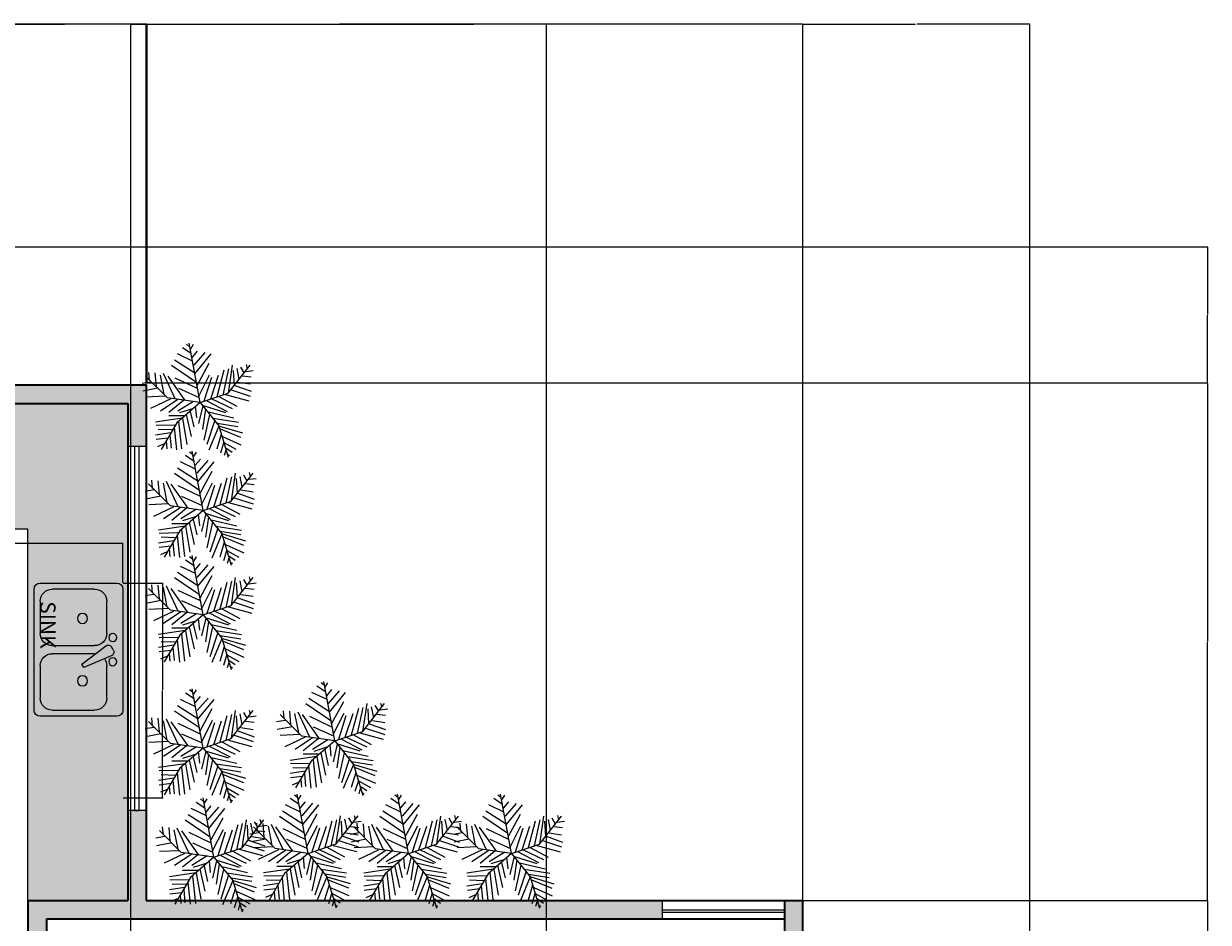
# Model space of a CAD drawing. Units: inches. Extents: x 192 to 1361, y -1362 to 367.
# Tile 23 of 23: x 783 to 1361, y -71 to 367. Entities that reach past the tile are written whole.
import ezdxf

# ---------------------------------------------------------------- set-up
doc = ezdxf.new("R2010")
doc.units = ezdxf.units.IN
doc.header["$MEASUREMENT"] = 0
for name, color, linetype, lineweight in [('A-ANNO-DIMS', 2, 'Continuous', 18), ('A-FLOR-CASE', 32, 'Continuous', 18), ('A-FLOR-FIXT', 8, 'Continuous', 18), ('A-WALL-PATT', 250, 'Continuous', 13), ('lawn', 96, 'Continuous', 13), ('text', 7, 'Continuous', 18), ('walls', 7, 'Continuous', 35), ('windows', 4, 'Continuous', 18)]:
    doc.layers.add(name, color=color, linetype=linetype, lineweight=lineweight)
doc.layers.add('A-FLOR-CASE-PATT', color=9, linetype='Continuous', lineweight=13, true_color=0xc7c8ca)
doc.layers.add('A-FLOR-FIXT-PATT', color=251, linetype='Continuous', lineweight=13, true_color=0x636466)
doc.styles.add('ATT', font='TXT')
doc.styles.get("Standard").update_dxf_attribs({"font": 'arial.ttf'})
doc.dimstyles.get("Standard").update_dxf_attribs({"dimtxt": 0.18, "dimasz": 0.18, "dimexe": 0.18, "dimexo": 0.0625, "dimgap": 0.09, "dimtad": 0, "dimtih": 1, "dimtoh": 1, "dimzin": 0, "dimdsep": 46, "dimlunit": 3, "dimtxsty": 'Standard', "dimcen": 0.09, "dimadec": 0, "dimazin": 0, "dimtfac": 1, "dimtofl": 0, "dimtmove": 0, "dimatfit": 3, "dimfxl": 1, "dimtolj": 1, "dimtzin": 0, "dimarcsym": 0})

# ---------------------------------------------------------------- blocks, each defined once
blk = doc.blocks.new('*U4')
for p, q in [((0, 0), (-10.5, 57)), ((-7.288, 39.707), (-21.778, 46.673)), ((-8.737, 47.138), (-17.069, 52.711)), ((-10.186, 53.64), (-13.084, 55.962)), ((-9.099, 51.782), (-6.563, 55.962)), ((-7.65, 43.423), (-2.578, 49.46)), ((-5.839, 35.992), (4.667, 48.067)), ((-5.114, 27.632), (10.463, 46.673)), ((-3.665, 19.273), (-27.574, 35.527)), ((-5.114, 28.097), (-24.676, 40.636)), ((-2.941, 16.486), (8.652, 37.85)), ((27, 9), (48, 36)), ((27.127, 9.056), (31.112, 35.992)), ((38.719, 34.134), (41.979, 28.561)), ((44.153, 36.456), (45.239, 32.741)), ((-31.5, 4.5), (-52.5, 25.5)), ((-48.585, 21.131), (-49.309, 29.026)), ((-43.513, 28.561), (-42.427, 15.558)), ((-38.442, 26.239), (-34.819, 7.663)), ((-35.544, 28.097), (-24.314, 3.947)), ((-14.533, 2.09), (-30.834, 25.31)), ((-24.314, 23.917), (-2.941, 13.7)), ((-1.129, 6.734), (9.014, 26.704)), ((3.942, 1.625), (11.187, 24.381)), ((10.101, 3.483), (17.708, 26.239)), ((16.259, 5.805), (23.142, 31.348)), ((22.055, 7.198), (27.489, 32.277)), ((31.836, 30.883), (32.561, 16.486)), ((35.096, 32.741), (37.27, 22.524)), ((40.53, 25.775), (48.862, 24.846)), ((43.791, 29.954), (51.036, 30.883)), ((-47.498, 19.737), (-55.83, 18.344)), ((-40.615, 13.7), (-55.105, 10.913)), ((-20.691, 13.7), (-1.129, 4.876)), ((29.662, 12.307), (48.137, 6.269)), ((33.285, 16.486), (48.862, 10.913)), ((36.183, 19.737), (48.137, 17.88)), ((-33.37, 6.269), (-52.207, 5.34)), ((-28.299, 3.483), (-47.86, -5.805)), ((-21.416, 3.018), (-38.079, -8.128)), ((0, 0), (-31.5, 4.5)), ((-15.982, 2.09), (-30.11, -9.521)), ((0, 0), (-22.5, -19.5)), ((-6.563, 1.161), (-21.416, -8.128)), ((0, 0), (27, 9)), ((0, 0), (18, -22.5)), ((6.478, 1.625), (26.04, -8.592)), ((11.187, 3.483), (30.749, -5.805)), ((18.07, 5.805), (35.096, -3.483)), ((24.229, 7.663), (46.688, 1.625)), ((-6.563, -5.805), (-19.967, -9.985)), ((-9.461, -8.592), (-6.201, -23.453)), ((-4.752, -3.483), (-3.665, -14.629)), ((2.493, -3.019), (-1.491, -20.202)), ((1.769, -2.555), (24.229, -9.521)), ((5.029, -6.27), (2.131, -25.775)), ((7.565, -9.056), (32.198, -14.629)), ((-17.431, -15.094), (-42.789, -18.809)), ((-24.314, -21.596), (-42.427, -22.06)), ((-22.5, -19.5), (-37.5, -45)), ((-15.257, -12.772), (-30.11, -12.772)), ((-20.691, -18.345), (-17.793, -44.352)), ((-17.069, -15.094), (-12.721, -40.172)), ((-13.446, -11.378), (-8.737, -32.741)), ((9.014, -11.378), (3.58, -35.992)), ((14.085, -16.951), (6.478, -40.172)), ((18.07, -22.524), (8.289, -45.745)), ((12.274, -15.094), (36.907, -18.809)), ((16.259, -19.738), (36.183, -22.989)), ((18, -22.5), (27, -52.5)), ((18.433, -22.524), (40.53, -29.026)), ((-28.299, -29.026), (-42.789, -31.348)), ((-26.849, -26.24), (-40.253, -25.775)), ((-29.023, -30.884), (-27.936, -43.887)), ((-25.038, -23.918), (-22.865, -45.281)), ((20.244, -30.419), (15.897, -44.816)), ((19.157, -25.311), (38.719, -33.206)), ((21.331, -32.741), (39.081, -40.636)), ((-30.834, -34.135), (-42.427, -35.528)), ((-34.457, -39.708), (-40.978, -42.494)), ((-32.646, -36.921), (-31.921, -44.352)), ((22.78, -37.85), (19.519, -48.532)), ((22.78, -38.314), (34.372, -44.816)), ((24.591, -43.423), (30.749, -47.603)), ((24.591, -45.745), (23.142, -50.854)), ((26.764, -49.925), (28.213, -50.854))]:
    blk.add_line(p, q)
blk = doc.blocks.new('15PSNK10')
at = {"color": 0, "linetype": 'ByBlock'}
for p, q in [((0, 15), (0, -15)), ((20.5, 16.5), (1.5, 16.5)), ((7, 15), (17.5, 15)), ((22, -15), (22, 15)), ((4, 4), (4, 12)), ((20.5, 12), (20.5, 4)), ((2.37, -0.1), (2.77, 0.6)), ((10.18, -3.57), (4.27, 0.87)), ((17.5, 1), (7, 1)), ((2.88, -1.54), (9.68, -4.43)), ((7.04, -1), (17.5, -1)), ((4, -12), (4, -4)), ((9.68, -4.43), (10.18, -3.57)), ((20.5, -4), (20.5, -12)), ((1.5, -16.5), (20.5, -16.5)), ((17.5, -15), (7, -15))]:
    blk.add_line(p, q, dxfattribs=at)
for centre, radius in [((10, 7.75), 1.25), ((2.5, 3), 1), ((2.5, -3), 1), ((10, -7.75), 1.25)]:
    blk.add_circle(centre, radius, dxfattribs=at)
for centre, radius, start, end in [((1.5, 15), 1.5, 90, 180), ((7, 12), 3, 90, 180), ((17.5, 12), 3, 0, 90), ((20.5, 15), 1.5, 0, 90), ((7, 4), 3, 180, 270), ((17.5, 4), 3, 270, 0), ((3.63, 0.1), 1, 50.5377, 150), ((3.23, -0.6), 1, 150, 249.4623), ((7, -4), 3, 146.607, 180), ((17.5, -4), 3, 0, 90), ((7, -12), 3, 180, 270), ((17.5, -12), 3, 270, 0), ((1.5, -15), 1.5, 180, 270), ((20.5, -15), 1.5, 270, 0)]:
    blk.add_arc(centre, radius, start, end, dxfattribs=at)
at = {"color": 0, "linetype": 'ByBlock', "style": 'ATT'}
for tag, p, flags in [('ITEM', (0, -26), 3), ('ROOM_NUMBER', (0, -35), 1)]:
    blk.add_attdef(tag, p, '', height=6, dxfattribs=dict(at, flags=flags))
blk = doc.blocks.new('*D45')
at = {"layer": 'A-ANNO-DIMS', "color": 0, "lineweight": -2, "transparency": 16777216}
for p, q in [((701.78, 94.46), (701.78, 113.98)), ((701.96, 113.8), (765.84, 113.8)), ((830.96, 113.8), (767.08, 113.8)), ((831.14, 94.46), (831.14, 113.98))]:
    blk.add_line(p, q, dxfattribs=at)
at = {"layer": 'A-ANNO-DIMS', "color": 0, "transparency": 16777216}
for points in [[(701.96, 113.83), (701.96, 113.77), (701.78, 113.8)], [(830.96, 113.83), (830.96, 113.77), (831.14, 113.8)]]:
    blk.add_solid(points, dxfattribs=at)
at = {"layer": 'Defpoints', "color": 0, "transparency": 16777216}
for p in [(701.78, 113.8), (701.78, 94.4), (831.14, 94.4)]:
    blk.add_point(p, dxfattribs=at)
at = {"layer": 'A-ANNO-DIMS', "color": 0, "transparency": 16777216, "insert": (766.46, 113.8), "char_height": 0.18, "attachment_point": 5}
blk.add_mtext('\\A1;SINK 129', dxfattribs=at)
blk = doc.blocks.new('*D46')
at = {"layer": 'A-ANNO-DIMS', "color": 0, "lineweight": -2, "transparency": 16777216}
for p, q in [((831.2, 94.4), (850.72, 94.4)), ((850.54, 94.22), (850.54, 42.23)), ((850.54, -10.13), (850.54, 41.86)), ((831.2, -10.31), (850.72, -10.31))]:
    blk.add_line(p, q, dxfattribs=at)
at = {"layer": 'A-ANNO-DIMS', "color": 0, "transparency": 16777216}
for points in [[(850.51, 94.22), (850.57, 94.22), (850.54, 94.4)], [(850.51, -10.13), (850.57, -10.13), (850.54, -10.31)]]:
    blk.add_solid(points, dxfattribs=at)
at = {"layer": 'Defpoints', "color": 0, "transparency": 16777216}
for p in [(831.14, 94.4), (850.54, 94.4), (831.14, -10.31)]:
    blk.add_point(p, dxfattribs=at)
at = {"layer": 'A-ANNO-DIMS', "color": 0, "transparency": 16777216, "insert": (850.54, 42.04), "char_height": 0.18, "attachment_point": 5}
blk.add_mtext('\\A1;105', dxfattribs=at)
blk = doc.blocks.new('*D50')
at = {"layer": 'A-ANNO-DIMS', "color": 0, "lineweight": -2, "transparency": 16777216}
for p, q in [((300.55, 191.16), (300.55, 367.39)), ((300.73, 367.21), (571.36, 367.21)), ((842.77, 367.21), (572.14, 367.21)), ((842.95, 192.11), (842.95, 367.39))]:
    blk.add_line(p, q, dxfattribs=at)
at = {"layer": 'A-ANNO-DIMS', "color": 0, "transparency": 16777216}
for points in [[(300.73, 367.24), (300.73, 367.18), (300.55, 367.21)], [(842.77, 367.24), (842.77, 367.18), (842.95, 367.21)]]:
    blk.add_solid(points, dxfattribs=at)
at = {"layer": 'Defpoints', "color": 0, "transparency": 16777216}
for p in [(842.95, 367.21), (300.55, 191.1), (842.95, 192.05)]:
    blk.add_point(p, dxfattribs=at)
at = {"layer": 'A-ANNO-DIMS', "color": 0, "transparency": 16777216, "insert": (571.75, 367.21), "char_height": 0.18, "attachment_point": 5}
blk.add_mtext('\\A1;542.4', dxfattribs=at)
blk = doc.blocks.new('*D51')
at = {"layer": 'A-ANNO-DIMS', "color": 0, "lineweight": -2, "transparency": 16777216}
for p, q in [((842.95, 192.11), (842.95, 367.39)), ((843.13, 367.21), (1002.41, 367.21)), ((1162.62, 367.21), (1003.34, 367.21)), ((1162.8, -60.44), (1162.8, 367.39))]:
    blk.add_line(p, q, dxfattribs=at)
at = {"layer": 'A-ANNO-DIMS', "color": 0, "transparency": 16777216}
for points in [[(843.13, 367.24), (843.13, 367.18), (842.95, 367.21)], [(1162.62, 367.24), (1162.62, 367.18), (1162.8, 367.21)]]:
    blk.add_solid(points, dxfattribs=at)
at = {"layer": 'Defpoints', "color": 0, "transparency": 16777216}
for p in [(1162.8, 367.21), (842.95, 192.05), (1162.8, -60.5)]:
    blk.add_point(p, dxfattribs=at)
at = {"layer": 'A-ANNO-DIMS', "color": 0, "transparency": 16777216, "insert": (1002.88, 367.21), "char_height": 0.18, "attachment_point": 5}
blk.add_mtext('\\A1;319.85', dxfattribs=at)
blk = doc.blocks.new('*D52')
at = {"layer": 'A-ANNO-DIMS', "color": 0, "lineweight": -2, "transparency": 16777216}
for p, q in [((1162.8, -60.44), (1162.8, 367.39)), ((1162.98, 367.21), (1217.73, 367.21)), ((1273.39, 367.21), (1218.64, 367.21)), ((1273.57, -597.44), (1273.57, 367.39))]:
    blk.add_line(p, q, dxfattribs=at)
at = {"layer": 'A-ANNO-DIMS', "color": 0, "transparency": 16777216}
for points in [[(1162.98, 367.24), (1162.98, 367.18), (1162.8, 367.21)], [(1273.39, 367.24), (1273.39, 367.18), (1273.57, 367.21)]]:
    blk.add_solid(points, dxfattribs=at)
at = {"layer": 'Defpoints', "color": 0, "transparency": 16777216}
for p in [(1273.57, 367.21), (1162.8, -60.5), (1273.57, -597.5)]:
    blk.add_point(p, dxfattribs=at)
at = {"layer": 'A-ANNO-DIMS', "color": 0, "transparency": 16777216, "insert": (1218.18, 367.21), "char_height": 0.18, "attachment_point": 5}
blk.add_mtext('\\A1;110.76', dxfattribs=at)
blk = doc.blocks.new('*D53')
at = {"layer": 'A-ANNO-DIMS', "color": 0, "lineweight": -2, "transparency": 16777216}
for p, q in [((534.69, 258.53), (1360.41, 258.53)), ((1360.23, 258.35), (1360.23, 225.47)), ((1360.23, 192.23), (1360.23, 225.11)), ((843.02, 192.05), (1360.41, 192.05))]:
    blk.add_line(p, q, dxfattribs=at)
at = {"layer": 'A-ANNO-DIMS', "color": 0, "transparency": 16777216}
for points in [[(1360.2, 258.35), (1360.26, 258.35), (1360.23, 258.53)], [(1360.2, 192.23), (1360.26, 192.23), (1360.23, 192.05)]]:
    blk.add_solid(points, dxfattribs=at)
at = {"layer": 'Defpoints', "color": 0, "transparency": 16777216}
for p in [(534.62, 258.53), (1360.23, 258.53), (842.95, 192.05)]:
    blk.add_point(p, dxfattribs=at)
at = {"layer": 'A-ANNO-DIMS', "color": 0, "transparency": 16777216, "insert": (1360.23, 225.29), "char_height": 0.18, "attachment_point": 5}
blk.add_mtext('\\A1;66.48', dxfattribs=at)
blk = doc.blocks.new('*D54')
at = {"layer": 'A-ANNO-DIMS', "color": 0, "lineweight": -2, "transparency": 16777216}
for p, q in [((843.02, 192.05), (1360.41, 192.05)), ((1360.23, 191.87), (1360.23, 65.96)), ((1360.23, -60.32), (1360.23, 65.59)), ((1162.87, -60.5), (1360.41, -60.5))]:
    blk.add_line(p, q, dxfattribs=at)
at = {"layer": 'A-ANNO-DIMS', "color": 0, "transparency": 16777216}
for points in [[(1360.2, 191.87), (1360.26, 191.87), (1360.23, 192.05)], [(1360.2, -60.32), (1360.26, -60.32), (1360.23, -60.5)]]:
    blk.add_solid(points, dxfattribs=at)
at = {"layer": 'Defpoints', "color": 0, "transparency": 16777216}
for p in [(842.95, 192.05), (1162.8, -60.5), (1360.23, -60.5)]:
    blk.add_point(p, dxfattribs=at)
at = {"layer": 'A-ANNO-DIMS', "color": 0, "transparency": 16777216, "insert": (1360.23, 65.77), "char_height": 0.18, "attachment_point": 5}
blk.add_mtext('\\A1;252.55', dxfattribs=at)
blk = doc.blocks.new('*D55')
at = {"layer": 'A-ANNO-DIMS', "color": 0, "lineweight": -2, "transparency": 16777216}
for p, q in [((1162.87, -60.5), (1360.41, -60.5)), ((1360.23, -60.68), (1360.23, -116.3)), ((1360.23, -172.29), (1360.23, -116.67)), ((1162.87, -172.47), (1360.41, -172.47))]:
    blk.add_line(p, q, dxfattribs=at)
at = {"layer": 'A-ANNO-DIMS', "color": 0, "transparency": 16777216}
for points in [[(1360.2, -60.68), (1360.26, -60.68), (1360.23, -60.5)], [(1360.2, -172.29), (1360.26, -172.29), (1360.23, -172.47)]]:
    blk.add_solid(points, dxfattribs=at)
at = {"layer": 'Defpoints', "color": 0, "transparency": 16777216}
for p in [(1162.8, -60.5), (1162.8, -172.47), (1360.23, -172.47)]:
    blk.add_point(p, dxfattribs=at)
at = {"layer": 'A-ANNO-DIMS', "color": 0, "transparency": 16777216, "insert": (1360.23, -116.49), "char_height": 0.18, "attachment_point": 5}
blk.add_mtext('\\A1;111.97', dxfattribs=at)
blk = doc.blocks.new('*D65')
at = {"layer": 'A-ANNO-DIMS', "color": 0, "lineweight": -2, "transparency": 16777216}
for p, q in [((763.44, 191.16), (763.44, 367.39)), ((763.62, 367.21), (802.69, 367.21)), ((842.37, 367.21), (803.3, 367.21)), ((842.55, 191.16), (842.55, 367.39))]:
    blk.add_line(p, q, dxfattribs=at)
at = {"layer": 'A-ANNO-DIMS', "color": 0, "transparency": 16777216}
for points in [[(763.62, 367.24), (763.62, 367.18), (763.44, 367.21)], [(842.37, 367.24), (842.37, 367.18), (842.55, 367.21)]]:
    blk.add_solid(points, dxfattribs=at)
at = {"layer": 'Defpoints', "color": 0, "transparency": 16777216}
for p in [(842.55, 367.21), (763.44, 191.1), (842.55, 191.1)]:
    blk.add_point(p, dxfattribs=at)
at = {"layer": 'A-ANNO-DIMS', "color": 0, "transparency": 16777216, "insert": (802.99, 367.21), "char_height": 0.18, "attachment_point": 5}
blk.add_mtext('\\A1;79.1', dxfattribs=at)
blk = doc.blocks.new('*D72')
at = {"layer": 'A-ANNO-DIMS', "color": 0, "lineweight": -2, "transparency": 16777216}
for p, q in [((835.08, -1067.56), (835.08, 367.39)), ((835.26, 367.21), (935.95, 367.21)), ((1037.58, 367.21), (936.88, 367.21)), ((1037.76, -1067.56), (1037.76, 367.39))]:
    blk.add_line(p, q, dxfattribs=at)
at = {"layer": 'A-ANNO-DIMS', "color": 0, "transparency": 16777216}
for points in [[(835.26, 367.24), (835.26, 367.18), (835.08, 367.21)], [(1037.58, 367.24), (1037.58, 367.18), (1037.76, 367.21)]]:
    blk.add_solid(points, dxfattribs=at)
at = {"layer": 'Defpoints', "color": 0, "transparency": 16777216}
for p in [(1037.76, 367.21), (835.08, -1067.62), (1037.76, -1067.62)]:
    blk.add_point(p, dxfattribs=at)
at = {"layer": 'A-ANNO-DIMS', "color": 0, "transparency": 16777216, "insert": (936.42, 367.21), "char_height": 0.18, "attachment_point": 5}
blk.add_mtext('\\A1;202.68', dxfattribs=at)

msp = doc.modelspace()

# ---------------------------------------------------------------- hatches: boundary and pattern name
at = {"layer": 'A-FLOR-CASE-PATT'}
h = msp.add_hatch(color=256, dxfattribs=at)
h.dxf.hatch_style = 1
h.paths.add_polyline_path([(833.5452, 182.102), (606.0353, 182.102), (606.0321, 180.6288), (606.1093, 180.6286), (606.0056, 120.6543), (784.8041, 120.6543), (784.8041, -60.4996), (833.5452, -60.4996)])
at = {"layer": 'A-FLOR-FIXT-PATT'}
h = msp.add_hatch(color=256, dxfattribs=at)
h.dxf.hatch_style = 1
h.paths.add_polyline_path([(831.1357, 91.4445, 0.41421356), (828.1842, 94.3961), (790.7977, 94.3961, 0.41421356), (787.8462, 91.4445), (787.8462, 32.4133, 0.41421356), (790.7977, 29.4617), (828.1842, 29.4617, 0.41421356), (831.1357, 32.4133)])
h.paths.add_polyline_path([(813.9183, 46.6791, -1), (808.999, 46.6791, -1)], flags=16)
h.paths.add_polyline_path([(811.108, 54.9101), (822.7336, 63.6427, -0.46319752), (825.6875, 63.1088), (826.4802, 61.7357, -0.46370743), (825.4673, 58.9078), (812.0919, 53.206)], flags=16)
h.paths.add_polyline_path([(796.7008, 63.8966, -0.41421356), (790.7977, 69.7997), (790.7977, 85.5414, -0.41421356), (796.7008, 91.4445), (817.3618, 91.4445, -0.41421356), (823.2649, 85.5414), (823.2649, 69.7997, -0.41421356), (817.3618, 63.8966)], flags=16)
h.paths.add_polyline_path([(824.2488, 56.0258, -1), (828.1842, 56.0258, -1)], flags=16)
h.paths.add_polyline_path([(808.999, 77.1786, -1), (813.9183, 77.1786, -1)], flags=0)
h.paths.add_polyline_path([(824.2488, 67.832, -1), (828.1842, 67.832, -1)], flags=16)
h.paths.add_polyline_path([(823.2649, 85.5414, 0.41421356), (817.3618, 91.4445), (796.7008, 91.4445, 0.41421356), (790.7977, 85.5414), (790.7977, 69.7997, 0.41421356), (796.7008, 63.8966), (817.3618, 63.8966, 0.41421356), (823.2649, 69.7997)], flags=0)
h = msp.add_hatch(color=256, dxfattribs=at)
h.dxf.hatch_style = 1
h.paths.add_polyline_path([(823.2649, 85.5414, 0.41421356), (817.3618, 91.4445), (796.7008, 91.4445, 0.41421356), (790.7977, 85.5414), (790.7977, 69.7997, 0.41421356), (796.7008, 63.8966), (817.3618, 63.8966, 0.41421356), (823.2649, 69.7997)])
h.paths.add_polyline_path([(808.999, 77.1786, -1), (813.9183, 77.1786, -1)], flags=16)
at = {"layer": 'A-WALL-PATT'}
h = msp.add_hatch(color=256, dxfattribs=at)
h.dxf.hatch_style = 1
h.paths.add_polyline_path([(309.5452, 191.102), (300.5452, 191.102), (300.5452, -126.898), (309.5452, -126.898), (309.5452, -117.898)])
h.paths.add_polyline_path([(420.798, 191.102), (337.3229, 191.102), (337.3229, 182.102), (420.798, 182.102)])
h.paths.add_polyline_path([(518.5452, 182.102), (625.4022, 182.102), (625.4022, 191.102), (509.5452, 191.102), (509.5452, 114.3262), (518.5452, 114.3262)])
h.paths.add_polyline_path([(842.5452, 191.102), (763.4438, 191.102), (763.4438, 182.102), (833.5452, 182.102), (833.5452, 161.1615), (836.8088, 161.1615), (842.5452, 161.1615)])
h.paths.add_polyline_path([(842.5452, -16.5675), (833.5452, -16.5675), (833.5452, -60.4996), (784.8041, -60.4996), (784.8041, -354.6796), (793.8041, -354.6796), (793.8041, -69.4996), (1094.1252, -69.4996), (1094.1252, -60.4996), (842.5452, -60.4996)])
h.paths.add_polyline_path([(518.5452, 36.602), (509.5452, 36.602), (509.5452, -117.898), (420.2204, -117.898), (420.2204, -126.898), (518.5452, -126.898)])
h.paths.add_polyline_path([(474.8041, -377.0384), (465.8041, -377.0384), (465.8041, -381.5384), (465.8041, -450.898), (537.5717, -450.898), (537.5717, -441.898), (474.8041, -441.898)])
h.paths.add_polyline_path([(1162.8041, -380.6763), (1204.3001, -380.6763), (1204.3001, -375.6763), (1195.1471, -375.6763), (1153.8041, -375.6763), (1153.8041, -448.4996), (856.5691, -448.4996), (856.5691, -457.4996), (1162.8041, -457.4996)])
h.paths.add_polyline_path([(1162.8041, -525.128), (1153.8041, -525.128), (1153.8041, -597.4996), (1162.8041, -597.4996)], flags=17)
h.paths.add_polyline_path([(1162.8041, -60.4996), (1153.8041, -60.4996), (1153.8041, -69.4996), (1153.8041, -177.4733), (1205.8889, -177.4733), (1205.8889, -172.4733), (1162.8041, -172.4733)])
h.paths.add_polyline_path([(980.5799, -525.686), (971.5799, -525.686), (971.5799, -597.4996), (980.5799, -597.4996)], flags=17)
h.paths.add_polyline_path([(856.5691, -448.4996), (798.7542, -448.4996), (784.8041, -448.4996), (784.8041, -457.4996), (847.5691, -457.4996), (847.5691, -597.4996), (784.8041, -597.4996), (784.8041, -606.4996), (1273.5658, -606.4996), (1273.5658, -597.4996), (856.5691, -597.4996)])
h.paths.add_polyline_path([(1273.5658, -773.892), (1099.8366, -773.892), (1099.8366, -851.9362), (1108.8366, -851.9362), (1108.8366, -782.892), (1273.5658, -782.892)])
h.paths.add_polyline_path([(1108.8366, -982.9214), (1099.8366, -982.9214), (1099.8366, -1067.6246), (1037.7563, -1067.6246), (1037.7563, -1076.6246), (1108.8366, -1076.6246)])
h.paths.add_polyline_path([(835.078, -1067.6246), (758.8458, -1067.6246), (758.8458, -940.2324), (749.8458, -940.2324), (749.8458, -963.172), (749.8458, -970.4644), (749.8458, -1076.6246), (835.078, -1076.6246)])
h.paths.add_polyline_path([(450.307, -1066.9838), (441.307, -1066.9838), (441.307, -1076.6246), (450.307, -1076.6246)])
h.paths.add_polyline_path([(492.8925, -756.4415), (274.8925, -756.4415), (274.8925, -765.4415), (492.8925, -765.4415)])
h.paths.add_polyline_path([(283.8925, -835.2244), (274.8925, -835.2244), (274.8925, -914.4415), (492.8925, -914.4415), (492.8925, -839.9415), (483.8925, -839.9415), (483.8925, -905.4415), (283.8925, -905.4415)])
h.paths.add_polyline_path([(283.8925, -441.898), (283.8925, -375.4296), (281.6021, -375.4296), (281.6021, -399.4121), (274.8925, -399.4121), (274.8925, -441.898), (274.8925, -684.5089), (283.8925, -684.5089)])

# ---------------------------------------------------------------- linework, layer by layer
at = {"layer": 'A-FLOR-CASE'}
for p, q in [((784.8041, 120.6543), (606.0056, 120.6543)), ((784.8041, -60.4996), (784.8041, 120.6543))]:
    msp.add_line(p, q, dxfattribs=at)
at = {"layer": 'walls'}
for p, q in [((504.3983, 191.102), (842.5452, 191.102)), ((842.5452, 191.102), (842.5452, -60.4996)), ((518.5452, 182.102), (833.5452, 182.102)), ((833.5452, 182.102), (833.5452, -60.4996)), ((784.8041, -60.4996), (784.8041, -354.6796)), ((784.8041, -60.4996), (833.5452, -60.4996)), ((842.5452, -60.4996), (1162.8041, -60.4996)), ((1153.8041, -60.4996), (1153.8041, -448.4996)), ((1162.8041, -172.4733), (1162.8041, -60.4996)), ((793.8041, -69.4996), (793.8041, -354.6796)), ((793.8041, -69.4996), (1153.8041, -69.4996))]:
    msp.add_line(p, q, dxfattribs=at)
at = {"layer": 'windows'}
for p, q in [((833.5452, 161.1615), (842.5452, 161.1615)), ((833.5452, 161.1615), (836.8088, 161.1615)), ((836.8088, 161.1615), (836.8088, -16.5675)), ((839.1278, -16.5675), (839.1278, 161.1615)), ((842.5452, -16.5675), (833.5452, -16.5675)), ((836.8088, -16.5675), (839.1278, -16.5675)), ((1094.1252, -60.4996), (1094.1252, -69.4996)), ((1153.8041, -60.4996), (1153.8041, -69.4996)), ((1094.1252, -64.9996), (1153.8041, -64.9996)), ((1094.1252, -66.1562), (1153.8041, -66.1562))]:
    msp.add_line(p, q, dxfattribs=at)

# ---------------------------------------------------------------- block references
at = {"layer": 'A-FLOR-FIXT', "xscale": -1.967708900679738, "yscale": 1.967708900679738, "zscale": 1.967708900679738}
msp.add_blockref('15PSNK10', (831.1357, 61.9289), dxfattribs=at)
at = {"layer": 'lawn', "xscale": 0.5078671948952364, "yscale": 0.5078671948952364, "zscale": 0.5078671948952364}
for p in [(868.8473, 182.4935), (870.3111, 129.8357), (870.3111, 78.8717), (934.4526, 17.3683), (870.3111, 13.9131), (875.5865, -39.3633), (921.4854, -37.4761), (970.4442, -37.5411), (1020.7144, -37.5411)]:
    msp.add_blockref('*U4', p, dxfattribs=at)

# ---------------------------------------------------------------- texts
at = {"layer": 'text'}
msp.add_text('SINK', height=7.5081, rotation=270, dxfattribs=at).set_placement((790.7977, 85.5414))

# ---------------------------------------------------------------- dimensions: what is measured, and where the dimension line sits
at = {"layer": 'A-ANNO-DIMS'}
for base, p1, p2, override, picture, middle in [((842.9527, 367.2097), (300.5452, 191.102), (842.9527, 192.0491), {"dimdec": 1, "dimlfac": 1, "dimrnd": 0, "dimzin": 0, "dimdsep": 46, "dimlunit": 2}, '*D50', (571.749, 367.2097)), ((842.5452, 367.2097), (763.4438, 191.102), (842.5452, 191.102), {"dimdec": 1, "dimlfac": 1, "dimrnd": 0, "dimzin": 0, "dimdsep": 46, "dimlunit": 2}, '*D65', (802.9945, 367.2097)), ((1037.7563, 367.2097), (835.078, -1067.6246), (1037.7563, -1067.6246), {"dimdec": 2, "dimlfac": 1, "dimrnd": 0, "dimzin": 0, "dimdsep": 46, "dimlunit": 2}, '*D72', (936.4171, 367.2097)), ((1162.8041, 367.2097), (842.9527, 192.0491), (1162.8041, -60.4996), {"dimdec": 2, "dimlfac": 1, "dimrnd": 0, "dimzin": 0, "dimdsep": 46, "dimlunit": 2}, '*D51', (1002.8784, 367.2097)), ((1273.5658, 367.2097), (1162.8041, -60.4996), (1273.5658, -597.4996), {"dimdec": 2, "dimlfac": 1, "dimrnd": 0, "dimzin": 0, "dimdsep": 46, "dimlunit": 2}, '*D52', (1218.185, 367.2097))]:
    dim = msp.add_linear_dim(base=base, p1=p1, p2=p2, dimstyle='Standard', override=override, dxfattribs=at)
    dim.commit()
    dim.dimension.update_dxf_attribs({"geometry": picture, "text_midpoint": middle})
for base, p1, p2, override, picture, middle in [((1360.2331, 258.5286), (842.9527, 192.0491), (534.6249, 258.5286), {"dimdec": 2, "dimlfac": 1, "dimrnd": 0, "dimzin": 0, "dimdsep": 46, "dimlunit": 2}, '*D53', (1360.2331, 225.2888)), ((1360.2331, -60.4996), (842.9527, 192.0491), (1162.8041, -60.4996), {"dimdec": 2, "dimlfac": 1, "dimrnd": 0, "dimzin": 0, "dimdsep": 46, "dimlunit": 2}, '*D54', (1360.2331, 65.7747)), ((850.539, 94.3961), (831.1357, -10.3096), (831.1357, 94.3961), {"dimdec": 0, "dimlfac": 1, "dimrnd": 0, "dimzin": 0, "dimdsep": 46, "dimlunit": 2}, '*D46', (850.539, 42.0432)), ((1360.2331, -172.4733), (1162.8041, -60.4996), (1162.8041, -172.4733), {"dimdec": 2, "dimlfac": 1, "dimrnd": 0, "dimzin": 0, "dimdsep": 46, "dimlunit": 2}, '*D55', (1360.2331, -116.4864))]:
    dim = msp.add_linear_dim(base=base, p1=p1, p2=p2, angle=90, dimstyle='Standard', override=override, dxfattribs=at)
    dim.commit()
    dim.dimension.update_dxf_attribs({"geometry": picture, "text_midpoint": middle})
dim = msp.add_linear_dim(base=(701.781, 113.7993), p1=(831.1357, 94.3961), p2=(701.781, 94.3961), angle=180, text='SINK <>', dimstyle='Standard', override={"dimdec": 0, "dimlfac": 1, "dimrnd": 0, "dimzin": 0, "dimdsep": 46, "dimlunit": 2}, dxfattribs=at)
dim.commit()
dim.dimension.update_dxf_attribs({"geometry": '*D45', "text_midpoint": (766.4584, 113.7993)})

doc.saveas('drawing.dxf')
